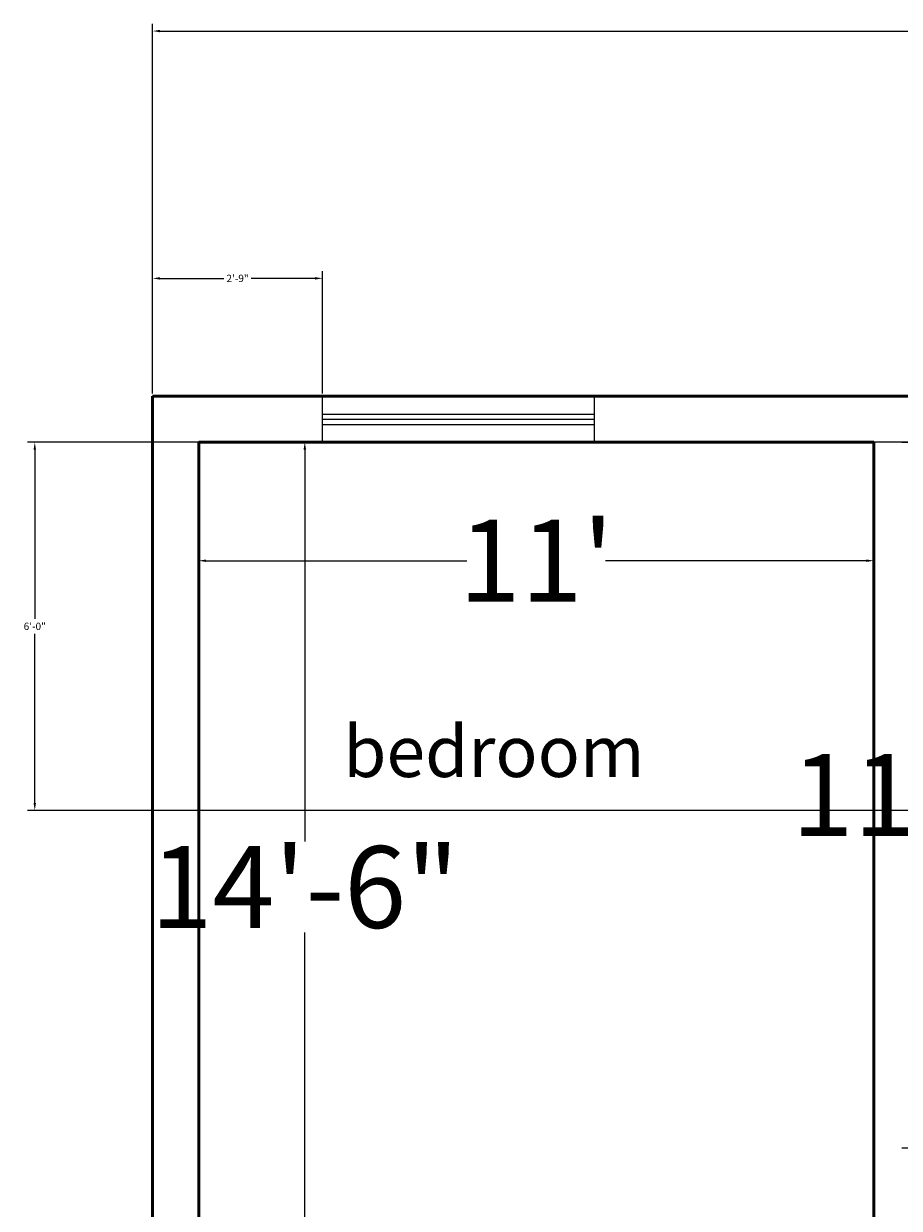
# Model space of a CAD drawing. Units: inches. Extents: x 325 to 804, y 366 to 834.
# Tile 2 of 6: x 325 to 496, y 603 to 834. Entities that reach past the tile are written whole.
import ezdxf

# ---------------------------------------------------------------- set-up
doc = ezdxf.new("R2010")
doc.units = ezdxf.units.IN
doc.header["$MEASUREMENT"] = 0
doc.layers.get('0').update_dxf_attribs({"color": 4})
for name, color, linetype, lineweight in [('A-ANNO-DIMS', 2, 'Continuous', 18), ('A-AREA-IDEN', 7, 'Continuous', 25), ('A-WALL', 7, 'Continuous', 50), ('window', 3, 'Continuous', 18)]:
    doc.layers.add(name, color=color, linetype=linetype, lineweight=lineweight)
doc.styles.get("Standard").update_dxf_attribs({"font": 'arial.ttf'})
doc.dimstyles.get("Standard").update_dxf_attribs({"dimscale": 8, "dimtxt": 0.18, "dimasz": 0.18, "dimexe": 0.18, "dimexo": 0.0625, "dimgap": 0.09, "dimtad": 0, "dimtih": 1, "dimtoh": 1, "dimdec": 0, "dimzin": 0, "dimdsep": 46, "dimlunit": 3, "dimtxsty": 'Standard', "dimcen": 0.09, "dimadec": 0, "dimazin": 0, "dimtfac": 1, "dimtdec": 0, "dimtofl": 0, "dimtmove": 0, "dimatfit": 3, "dimfxl": 1, "dimtolj": 1, "dimtzin": 0, "dimarcsym": 0})

# ---------------------------------------------------------------- blocks, each defined once
blk = doc.blocks.new('*D9')
at = {"layer": 'A-ANNO-DIMS', "color": 0, "lineweight": -2, "transparency": 16777216}
for p, q in [((359.97, 752.54), (381.66, 752.54)), ((380.22, 751.1), (380.22, 674.43)), ((380.22, 579.98), (380.22, 656.65)), ((359.97, 578.54), (381.66, 578.54))]:
    blk.add_line(p, q, dxfattribs=at)
at = {"layer": 'A-ANNO-DIMS', "color": 0, "transparency": 16777216}
for points in [[(379.98, 751.1), (380.46, 751.1), (380.22, 752.54)], [(379.98, 579.98), (380.46, 579.98), (380.22, 578.54)]]:
    blk.add_solid(points, dxfattribs=at)
at = {"layer": 'Defpoints', "color": 0, "transparency": 16777216}
for p in [(359.47, 752.54), (359.47, 578.54), (380.22, 578.54)]:
    blk.add_point(p, dxfattribs=at)
at = {"layer": 'A-ANNO-DIMS', "color": 0, "transparency": 16777216, "insert": (380.22, 665.54), "char_height": 1.44, "attachment_point": 5}
blk.add_mtext('\\A1;{\\H11.11111x;14\'-6"}', dxfattribs=at)
blk = doc.blocks.new('*D10')
at = {"layer": 'A-ANNO-DIMS', "color": 0, "lineweight": -2, "transparency": 16777216}
for p, q in [((359.47, 752.04), (359.47, 727.93)), ((491.47, 752.04), (491.47, 727.93)), ((360.91, 729.37), (411.93, 729.37)), ((490.03, 729.37), (439.02, 729.37))]:
    blk.add_line(p, q, dxfattribs=at)
at = {"layer": 'A-ANNO-DIMS', "color": 0, "transparency": 16777216}
for points in [[(360.91, 729.61), (360.91, 729.13), (359.47, 729.37)], [(490.03, 729.61), (490.03, 729.13), (491.47, 729.37)]]:
    blk.add_solid(points, dxfattribs=at)
at = {"layer": 'Defpoints', "color": 0, "transparency": 16777216}
for p in [(359.47, 752.54), (491.47, 752.54), (491.47, 729.37)]:
    blk.add_point(p, dxfattribs=at)
at = {"layer": 'A-ANNO-DIMS', "color": 0, "transparency": 16777216, "insert": (425.47, 729.37), "char_height": 1.44, "attachment_point": 5}
blk.add_mtext("\\A1;{\\H11.11111x;11'}", dxfattribs=at)
blk = doc.blocks.new('*D12')
at = {"layer": 'A-ANNO-DIMS', "color": 0, "lineweight": -2, "transparency": 16777216}
for p, q in [((496.97, 752.54), (507, 752.54)), ((505.56, 751.1), (505.56, 692.43)), ((505.56, 615.98), (505.56, 674.65)), ((496.97, 614.54), (507, 614.54))]:
    blk.add_line(p, q, dxfattribs=at)
at = {"layer": 'A-ANNO-DIMS', "color": 0, "transparency": 16777216}
for points in [[(505.32, 751.1), (505.8, 751.1), (505.56, 752.54)], [(505.32, 615.98), (505.8, 615.98), (505.56, 614.54)]]:
    blk.add_solid(points, dxfattribs=at)
at = {"layer": 'Defpoints', "color": 0, "transparency": 16777216}
for p in [(496.47, 752.54), (505.56, 752.54), (496.47, 614.54)]:
    blk.add_point(p, dxfattribs=at)
at = {"layer": 'A-ANNO-DIMS', "color": 0, "transparency": 16777216, "insert": (505.56, 683.54), "char_height": 1.44, "attachment_point": 5}
blk.add_mtext('\\A1;{\\H11.11111x;11\'-6"}', dxfattribs=at)
blk = doc.blocks.new('*D25')
at = {"layer": 'A-ANNO-DIMS', "color": 0, "lineweight": -2, "transparency": 16777216}
for p, q in [((350.47, 762.04), (350.47, 834.4)), ((774.47, 762.04), (774.47, 834.4)), ((351.91, 832.96), (559.28, 832.96)), ((773.03, 832.96), (565.67, 832.96))]:
    blk.add_line(p, q, dxfattribs=at)
at = {"layer": 'A-ANNO-DIMS', "color": 0, "transparency": 16777216}
for points in [[(351.91, 833.2), (351.91, 832.72), (350.47, 832.96)], [(773.03, 833.2), (773.03, 832.72), (774.47, 832.96)]]:
    blk.add_solid(points, dxfattribs=at)
at = {"layer": 'Defpoints', "color": 0, "transparency": 16777216}
for p in [(774.47, 832.96), (350.47, 761.54), (774.47, 761.54)]:
    blk.add_point(p, dxfattribs=at)
at = {"layer": 'A-ANNO-DIMS', "color": 0, "transparency": 16777216, "insert": (562.47, 832.96), "char_height": 1.44, "attachment_point": 5}
blk.add_mtext('\\A1;35\'-4"', dxfattribs=at)
blk = doc.blocks.new('WIN-53_14x9')
for p, q in [((0, 5.5), (53.14, 5.5)), ((0, 4.5), (53.14, 4.5)), ((0, 3.5), (53.14, 3.5))]:
    blk.add_line(p, q)
blk.add_lwpolyline([(0, 9), (53.14, 9), (53.14, 0), (0, 0)], close=True)
blk = doc.blocks.new('*D30')
at = {"layer": 'A-ANNO-DIMS', "color": 0, "lineweight": -2, "transparency": 16777216}
for p, q in [((350.47, 762.04), (350.47, 786.03)), ((383.67, 762.04), (383.67, 786.03)), ((351.91, 784.59), (364.42, 784.59)), ((382.23, 784.59), (369.72, 784.59))]:
    blk.add_line(p, q, dxfattribs=at)
at = {"layer": 'A-ANNO-DIMS', "color": 0, "transparency": 16777216}
for points in [[(351.91, 784.83), (351.91, 784.35), (350.47, 784.59)], [(382.23, 784.83), (382.23, 784.35), (383.67, 784.59)]]:
    blk.add_solid(points, dxfattribs=at)
at = {"layer": 'Defpoints', "color": 0, "transparency": 16777216}
for p in [(383.67, 784.59), (350.47, 761.54), (383.67, 761.54)]:
    blk.add_point(p, dxfattribs=at)
at = {"layer": 'A-ANNO-DIMS', "color": 0, "transparency": 16777216, "insert": (367.07, 784.59), "char_height": 1.44, "attachment_point": 5}
blk.add_mtext('\\A1;2\'-9"', dxfattribs=at)
blk = doc.blocks.new('*D37')
at = {"layer": 'A-ANNO-DIMS', "color": 0, "lineweight": -2, "transparency": 16777216}
for p, q in [((627.97, 752.54), (325.98, 752.54)), ((327.42, 751.1), (327.42, 717.99)), ((327.42, 681.98), (327.42, 715.08)), ((627.97, 680.54), (325.98, 680.54))]:
    blk.add_line(p, q, dxfattribs=at)
at = {"layer": 'A-ANNO-DIMS', "color": 0, "transparency": 16777216}
for points in [[(327.18, 751.1), (327.66, 751.1), (327.42, 752.54)], [(327.18, 681.98), (327.66, 681.98), (327.42, 680.54)]]:
    blk.add_solid(points, dxfattribs=at)
at = {"layer": 'Defpoints', "color": 0, "transparency": 16777216}
for p in [(327.42, 752.54), (628.47, 752.54), (628.47, 680.54)]:
    blk.add_point(p, dxfattribs=at)
at = {"layer": 'A-ANNO-DIMS', "color": 0, "transparency": 16777216, "insert": (327.42, 716.54), "char_height": 1.44, "attachment_point": 5}
blk.add_mtext('\\A1;6\'-0"', dxfattribs=at)

msp = doc.modelspace()

# ---------------------------------------------------------------- linework, layer by layer
at = {"layer": 'A-WALL'}
for p, q in [((350.47, 761.54), (774.47, 761.54)), ((350.47, 391.54), (350.47, 761.54)), ((359.47, 752.54), (491.47, 752.54)), ((359.47, 578.54), (359.47, 752.54)), ((491.47, 584.54), (491.47, 752.54))]:
    msp.add_line(p, q, dxfattribs=at)

# ---------------------------------------------------------------- block references
at = {"layer": 'window'}
msp.add_blockref('WIN-53_14x9', (383.67, 752.54), dxfattribs=at)

# ---------------------------------------------------------------- texts
at = {"layer": 'A-AREA-IDEN', "insert": (387.75, 697.06), "char_height": 10, "attachment_point": 1}
msp.add_mtext_dynamic_manual_height_columns('bedroom', width=79.8504, gutter_width=1, heights=[0], dxfattribs=at)

# ---------------------------------------------------------------- dimensions: what is measured, and where the dimension line sits
at = {"layer": 'A-ANNO-DIMS'}
for base, p2, override, picture, middle in [((774.47, 832.96), (774.47, 761.54), {"dimclrd": 0, "dimclre": 0, "dimclrt": 0}, '*D25', (562.47, 832.96)), ((383.67, 784.59), (383.67, 761.54), {"dimdec": 1, "dimlfac": 1, "dimrnd": 0, "dimzin": 1, "dimdsep": 46, "dimlunit": 4, "dimfrac": 2}, '*D30', (367.07, 784.59))]:
    dim = msp.add_linear_dim(base=base, p1=(350.47, 761.54), p2=p2, dimstyle='Standard', override=override, dxfattribs=at)
    dim.commit()
    dim.dimension.update_dxf_attribs({"geometry": picture, "text_midpoint": middle})
dim = msp.add_linear_dim(base=(327.42, 752.54), p1=(628.47, 680.54), p2=(628.47, 752.54), angle=90, dimstyle='Standard', override={"dimdec": 1, "dimlfac": 1, "dimrnd": 0, "dimzin": 1, "dimdsep": 46, "dimlunit": 4, "dimfrac": 2}, dxfattribs=at)
dim.commit()
dim.dimension.update_dxf_attribs({"geometry": '*D37', "text_midpoint": (327.42, 716.54)})
for base, p1, p2, picture, middle in [((380.22, 578.54), (359.47, 752.54), (359.47, 578.54), '*D9', (380.22, 665.54)), ((505.56, 752.54), (496.47, 614.54), (496.47, 752.54), '*D12', (505.56, 683.54))]:
    dim = msp.add_linear_dim(base=base, p1=p1, p2=p2, angle=90, text='{\\H11.11111x;<>}', dimstyle='Standard', override={"dimclrd": 0, "dimclre": 0, "dimclrt": 0}, dxfattribs=at)
    dim.commit()
    dim.dimension.update_dxf_attribs({"geometry": picture, "text_midpoint": middle})
dim = msp.add_linear_dim(base=(491.47, 729.37), p1=(359.47, 752.54), p2=(491.47, 752.54), text='{\\H11.11111x;<>}', dimstyle='Standard', override={"dimclrd": 0, "dimclre": 0, "dimclrt": 0}, dxfattribs=at)
dim.commit()
dim.dimension.update_dxf_attribs({"geometry": '*D10', "text_midpoint": (425.47, 729.37)})

doc.saveas('drawing.dxf')
